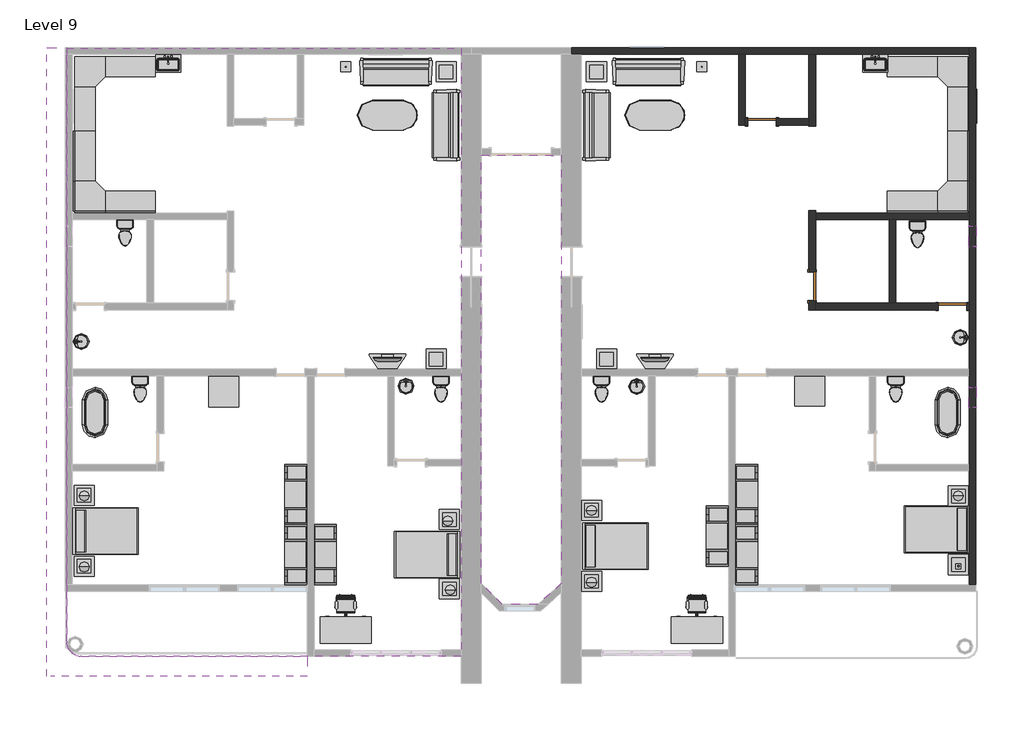
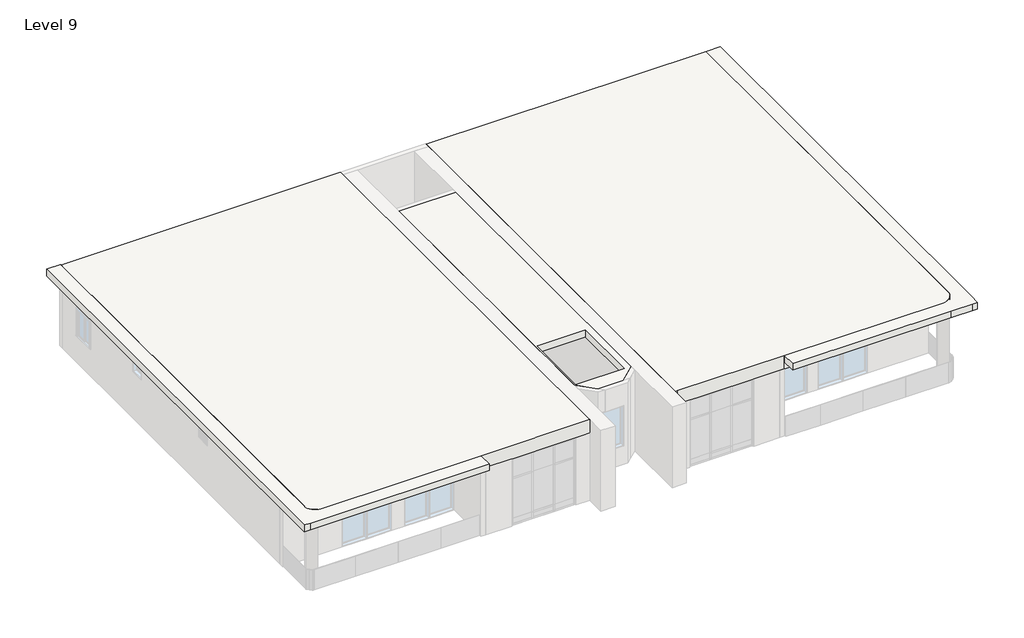
# One storey, part 3 of 3: 42 furniture elements, 14 flow terminals, 10 light fixtures, 9 walls, 3 doors, 3 slabs, 3 windows.
# Revit data of these elements (continued)
# Elements 40, 41 (IfcFurniture, "TV Stand : TV Stand") (continued)
#   Phase Created = New Construction
#   Materials on its faces: "Melamine - Gray", "Glass - Shelves"
# Elements 42, 43, 44, 45, 46, 47, 48, 49, 50, 51, 52, 53 (IfcFurniture, "Table-Coffee : 24\" x 24\" x 24\"")
#   Phase Created = New Construction
#   Materials on its faces: "Glass - Clear, Grey"
# Elements 54, 55 (IfcFurniture, "Table-Dining Oval : 36\" x 72\"")
#   Phase Created = New Construction
#   Materials on its faces: "Steel, Chrome Plated", "Glass - Clear, Grey"
# Elements 56, 57 (IfcFurniture, "Table-Rectangular : 36\" x 36\"")
#   Phase Created = New Construction
#   Materials on its faces: "Birch"
# Elements 58, 59 (IfcFurniture, "Work Station Cubicle : 96\" x 96\"")
#   Phase Created = New Construction
#   Materials on its faces: "Textile - Light Gray", "Laminate, Ivory, Matte"
# Element 60 (IfcLightFixture, "100W - 120V")
#   Mark = "104"
#   Phase Created = New Construction
#   Materials on its faces: "Steel, Chrome Plated", "Glass, Frosted"
# Element 61 (IfcLightFixture, "100W - 120V")
#   Mark = "105"
#   Phase Created = New Construction
#   Materials on its faces: "Steel, Chrome Plated", "Glass, Frosted"
# Element 62 (IfcLightFixture, "Table Lamp - Hemispheric : 60W - 120V")
#   Mark = "106"
#   Phase Created = New Construction
#   Materials on its faces: "Steel, Chrome Plated", "Glass, Frosted", "Birch"
# Element 63 (IfcLightFixture, "Table Lamp - Hemispheric : 60W - 120V")
#   Mark = "107"
#   Phase Created = New Construction
#   Materials on its faces: "Steel, Chrome Plated", "Glass, Frosted", "Birch"
# Element 64 (IfcLightFixture, "Table Lamp - Hemispheric : 60W - 120V")
#   Mark = "108"
#   Phase Created = New Construction
#   Materials on its faces: "Steel, Chrome Plated", "Glass, Frosted", "Birch"
# Element 65 (IfcLightFixture, "Table Lamp - Hemispheric : 60W - 120V")
#   Mark = "109"
#   Phase Created = New Construction
#   Materials on its faces: "Steel, Chrome Plated", "Glass, Frosted", "Birch"
# Element 66 (IfcLightFixture, "Table Lamp - Hemispheric : 60W - 120V")
#   Mark = "110"
#   Phase Created = New Construction
#   Materials on its faces: "Steel, Chrome Plated", "Glass, Frosted", "Birch"
# Element 67 (IfcLightFixture, "Table Lamp - Hemispheric : 60W - 120V")
#   Mark = "111"
#   Phase Created = New Construction
#   Materials on its faces: "Steel, Chrome Plated", "Glass, Frosted", "Birch"
# Element 68 (IfcLightFixture, "Table Lamp - Hemispheric : 60W - 120V")
#   Mark = "112"
#   Phase Created = New Construction
#   Materials on its faces: "Steel, Chrome Plated", "Glass, Frosted", "Birch"
# Element 69 (IfcLightFixture, "Table Lamp - Hemispheric : 60W - 120V")
#   Mark = "113"
#   Phase Created = New Construction
#   Materials on its faces: "Steel, Chrome Plated", "Glass, Frosted", "Birch"
# Element 70 (IfcSlab, "Generic - 12\" cream")
#   Height Offset From Level = 12' - 0"
#   Phase Created = New Construction
#   Materials on its faces: "Parking Stripe"
# Element 71 (IfcSlab, "Generic - 12\" white")
#   built-in parameter 1001955 = 3.14159 (stored number, unit not read)
#   Height Offset From Level = 12' - 0"
#   Phase Created = New Construction
#   Materials on its faces: "Door - Frame"
# Element 72 (IfcSlab, "Generic - 12\" white")
#   Height Offset From Level = 12' - 0"
#   Phase Created = New Construction
#   Materials on its faces: "Door - Frame"
# Elements 73, 74, 75, 76, 77, 78, 79, 80 (IfcWall, "Generic - 8\" cream")
#   Top Offset = 0' - 0"
#   Base Offset = 0' - 0"
#   Unconnected Height = 10' - 0"
#   wall height = 10' - 0"
#   Phase Created = New Construction
#   Base Constraint = Level 9
#   Materials on its faces: "Parking Stripe"
# Element 81 (IfcWall, "Generic - 8\" white")
#   Top Offset = 0' - 0"
#   Base Offset = 0' - 0"
#   Unconnected Height = 10' - 0"
#   wall height = 10' - 0"
#   Phase Created = New Construction
#   Base Constraint = Level 9
#   Materials on its faces: "Door - Frame", "Parking Stripe"
# Element 82 (IfcWindow, "Louvers with Trim : 24\" x 24\"")
#   Mark = "205"
#   Phase Created = New Construction
#   Materials on its faces: "Glass", "Iron, Ductile"
# Element 83 (IfcWindow, "Louvers with Trim : 24\" x 24\"")
#   Mark = "206"
#   Phase Created = New Construction
#   Materials on its faces: "Glass", "Iron, Ductile"
# Element 84 (IfcWindow, "Slider with Trim : 36\" x 48\"")
#   Mark = "202"
#   Phase Created = New Construction
#   Materials on its faces: "Iron, Ductile", "Glass"
# Materials
#   "Wood - Birch - Solid Stained Light Low Gloss": class "Wood", colour RGB 210 159 95, transparency 0, Cost = 0
#   "Paint - Sienna": colour RGB 118 70 51, transparency 0, Cost = 0
#   "Steel, Polished": class "Metal", colour RGB 57 57 57, transparency 0, Description = "Polished steel", Cost = 0
#   "Porcelain, Linen": class "Ceramic", colour RGB 249 239 230, transparency 0, Description = "Porcelain, linen", Cost = 0
#   "Laminate, Linen, Matte": class "Plastic", colour RGB 249 239 230, transparency 0, Description = "Plastic Laminate - Linen, Matte", Cost = 0
#   "Porcelain, Ivory": class "Ceramic", colour RGB 247 247 239, transparency 0, Description = "Porcelain, ivory", Cost = 0
#   "Laminate, Ivory, Matte": class "Plastic", colour RGB 247 247 239, transparency 0, Description = "Plastic Laminate - Ivory, Matte", Cost = 0
#   "Birch": class "Wood", colour RGB 224 178 126, transparency 0, Description = "Betula Alleghaniensis", Cost = 0
#   "Linen, White": class "Textile", colour RGB 247 247 239, transparency 0, Description = "Linen, white", Cost = 0
#   "Plastic, Opaque Black": class "Plastic", colour RGB 0 0 0, transparency 0.7, Description = "Plastic, generic, opaque black", Cost = 0
#   "Textile - Slate Blue": class "Fabric", colour RGB 98 102 118, transparency 0
#   "Steel, Chrome Plated": class "Metal", colour RGB 17 17 17, transparency 0, Description = "Chromiuim plated steel", Cost = 0
#   "Cherry": class "Wood", colour RGB 226 177 128, transparency 0, Description = "Prunus Serotina", Cost = 0
#   "Linen, Beige": class "Textile", colour RGB 249 239 230, transparency 0, Description = "Linen, beige", Cost = 0
#   "Melamine - Gray": class "Wood", colour RGB 49 49 49, transparency 0
#   "Glass - Clear, Grey": class "Glass", colour RGB 252 255 255, transparency 0.64
#   "Textile - Light Gray": class "Fabric", colour RGB 204 204 204, transparency 0
#   "Glass, Frosted": class "Glass", colour RGB 250 244 225, transparency 0.55, Description = "physical material", Cost = 0
#   "Parking Stripe": class "Paint", colour RGB 250 250 91, transparency 0, Cost = 0
#   "Door - Frame": colour RGB 118 70 51, transparency 0, Cost = 0
#   "Iron, Ductile": class "Metal", colour RGB 0 0 0, transparency 0, Description = "Ductile cast iron", Cost = 0
#   "Glass": class "Glass", colour RGB 0 128 192, transparency 0.75, Description = "Soda Lime Glass", Cost = 0
#   "TV - Black": colour RGB 49 49 49, transparency 0
#   "TV - Glass": colour RGB 157 157 157, transparency 0.9
#   "TV - Screen": colour RGB 0 0 0, transparency 0
#   "Glass - Shelves": class "Glass", colour RGB 167 167 167, transparency 0.9
